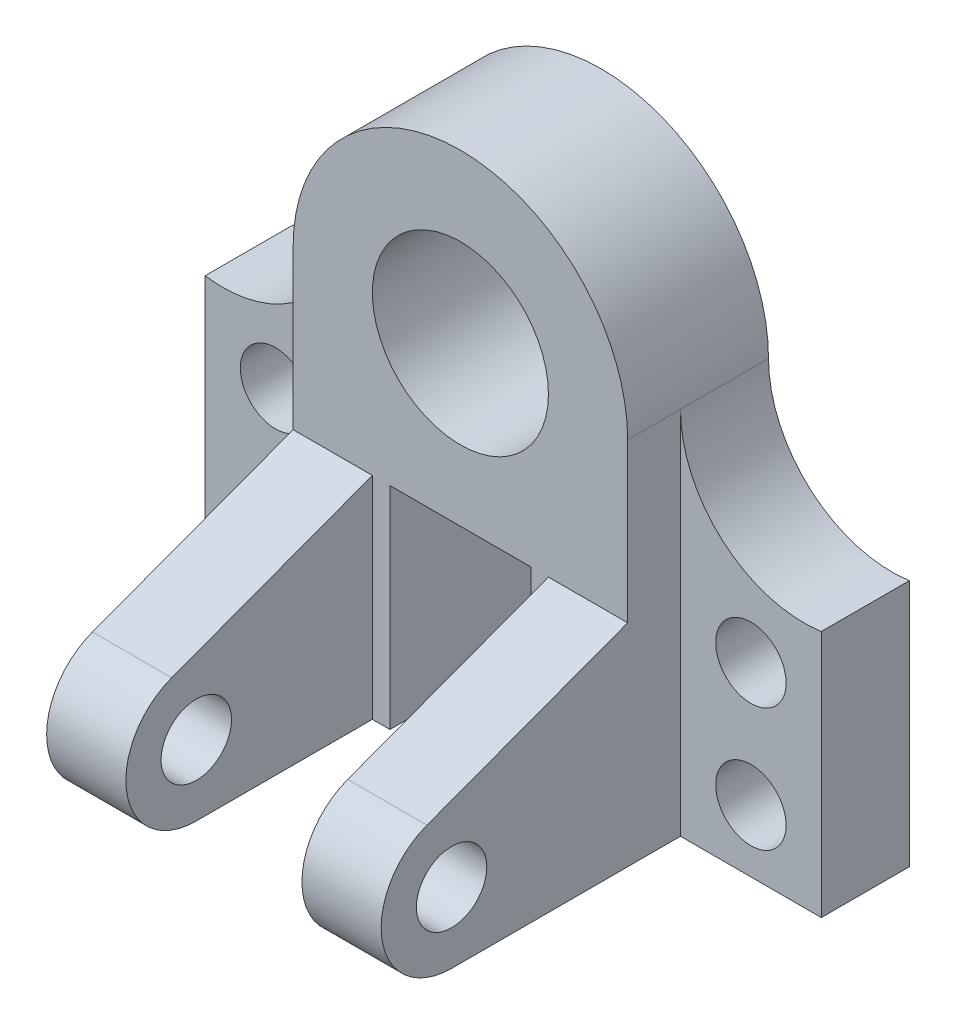
ISO-10303-21;
HEADER;
FILE_DESCRIPTION(('STEP AP214'),'2;1');
FILE_NAME('part.step','',(''),(''),'','','');
FILE_SCHEMA(('AUTOMOTIVE_DESIGN { 1 0 10303 214 1 1 1 1 }'));
ENDSEC;
DATA;
#1=APPLICATION_CONTEXT('core data for automotive mechanical design processes');
#2=APPLICATION_PROTOCOL_DEFINITION('international standard','automotive_design',2000,#1);
#3=PRODUCT_CONTEXT('',#1,'mechanical');
#4=PRODUCT('Part','Part','',(#3));
#5=PRODUCT_RELATED_PRODUCT_CATEGORY('part','',(#4));
#6=PRODUCT_DEFINITION_FORMATION('','',#4);
#7=PRODUCT_DEFINITION_CONTEXT('part definition',#1,'design');
#8=PRODUCT_DEFINITION('design','',#6,#7);
#9=PRODUCT_DEFINITION_SHAPE('','',#8);
#10=(LENGTH_UNIT() NAMED_UNIT(*) SI_UNIT(.MILLI.,.METRE.));
#11=(NAMED_UNIT(*) PLANE_ANGLE_UNIT() SI_UNIT($,.RADIAN.));
#12=(NAMED_UNIT(*) SI_UNIT($,.STERADIAN.) SOLID_ANGLE_UNIT());
#13=UNCERTAINTY_MEASURE_WITH_UNIT(LENGTH_MEASURE(1.E-05),#10,'distance_accuracy_value','');
#14=(GEOMETRIC_REPRESENTATION_CONTEXT(3) GLOBAL_UNCERTAINTY_ASSIGNED_CONTEXT((#13)) GLOBAL_UNIT_ASSIGNED_CONTEXT((#10,
#11,#12)) REPRESENTATION_CONTEXT('',''));
#15=CARTESIAN_POINT('',(0.,0.,0.));
#16=DIRECTION('',(0.,0.,1.));
#17=DIRECTION('',(1.,0.,0.));
#18=AXIS2_PLACEMENT_3D('',#15,#16,#17);
#19=CARTESIAN_POINT('',(-38.,-84.,32.));
#20=DIRECTION('',(0.,1.,0.));
#21=DIRECTION('',(0.,0.,1.));
#22=AXIS2_PLACEMENT_3D('',#19,#20,#21);
#23=PLANE('',#22);
#24=DIRECTION('',(1.,0.,0.));
#25=VECTOR('',#24,1.);
#26=CARTESIAN_POINT('',(-38.,-84.,0.));
#27=LINE('',#26,#25);
#28=CARTESIAN_POINT('',(-70.,-84.,0.));
#29=VERTEX_POINT('',#28);
#30=CARTESIAN_POINT('',(-16.,-84.,0.));
#31=VERTEX_POINT('',#30);
#32=EDGE_CURVE('E192',#29,#31,#27,.T.);
#33=ORIENTED_EDGE('',*,*,#32,.T.);
#34=DIRECTION('',(0.,0.,1.));
#35=VECTOR('',#34,1.);
#36=CARTESIAN_POINT('',(-16.,-84.,0.));
#37=LINE('',#36,#35);
#38=CARTESIAN_POINT('',(-16.,-84.,32.));
#39=VERTEX_POINT('',#38);
#40=EDGE_CURVE('E176',#31,#39,#37,.T.);
#41=ORIENTED_EDGE('',*,*,#40,.T.);
#42=DIRECTION('',(1.,0.,0.));
#43=VECTOR('',#42,1.);
#44=CARTESIAN_POINT('',(-38.,-84.,32.));
#45=LINE('',#44,#43);
#46=CARTESIAN_POINT('',(-20.,-84.,32.));
#47=VERTEX_POINT('',#46);
#48=EDGE_CURVE('E257',#47,#39,#45,.T.);
#49=ORIENTED_EDGE('',*,*,#48,.F.);
#50=DIRECTION('',(0.,0.,1.));
#51=VECTOR('',#50,1.);
#52=CARTESIAN_POINT('',(-20.,-84.,72.));
#53=LINE('',#52,#51);
#54=CARTESIAN_POINT('',(-20.,-84.,72.));
#55=VERTEX_POINT('',#54);
#56=EDGE_CURVE('E282',#47,#55,#53,.T.);
#57=ORIENTED_EDGE('',*,*,#56,.T.);
#58=DIRECTION('',(-1.,0.,0.));
#59=VECTOR('',#58,1.);
#60=CARTESIAN_POINT('',(-20.,-84.,72.));
#61=LINE('',#60,#59);
#62=CARTESIAN_POINT('',(-38.,-84.,72.));
#63=VERTEX_POINT('',#62);
#64=EDGE_CURVE('E223',#55,#63,#61,.T.);
#65=ORIENTED_EDGE('',*,*,#64,.T.);
#66=DIRECTION('',(0.,0.,-1.));
#67=VECTOR('',#66,1.);
#68=CARTESIAN_POINT('',(-38.,-84.,32.));
#69=LINE('',#68,#67);
#70=CARTESIAN_POINT('',(-38.,-84.,20.));
#71=VERTEX_POINT('',#70);
#72=EDGE_CURVE('E55',#63,#71,#69,.T.);
#73=ORIENTED_EDGE('',*,*,#72,.T.);
#74=DIRECTION('',(-1.,0.,0.));
#75=VECTOR('',#74,1.);
#76=CARTESIAN_POINT('',(-38.,-84.,20.));
#77=LINE('',#76,#75);
#78=CARTESIAN_POINT('',(-70.,-84.,20.));
#79=VERTEX_POINT('',#78);
#80=EDGE_CURVE('E218',#71,#79,#77,.T.);
#81=ORIENTED_EDGE('',*,*,#80,.T.);
#82=DIRECTION('',(0.,0.,-1.));
#83=VECTOR('',#82,1.);
#84=CARTESIAN_POINT('',(-70.,-84.,20.));
#85=LINE('',#84,#83);
#86=EDGE_CURVE('E200',#79,#29,#85,.T.);
#87=ORIENTED_EDGE('',*,*,#86,.T.);
#88=EDGE_LOOP('',(#33,#41,#49,#57,#65,#73,#81,#87));
#89=FACE_BOUND('',#88,.T.);
#90=ADVANCED_FACE('F43',(#89),#23,.F.);
#91=CARTESIAN_POINT('',(-38.,0.,32.));
#92=DIRECTION('',(1.,0.,0.));
#93=DIRECTION('',(0.,1.,0.));
#94=AXIS2_PLACEMENT_3D('',#91,#92,#93);
#95=PLANE('',#94);
#96=CARTESIAN_POINT('',(-38.,-68.,72.));
#97=DIRECTION('',(-1.,0.,0.));
#98=DIRECTION('',(0.,-1.,0.));
#99=AXIS2_PLACEMENT_3D('',#96,#97,#98);
#100=CIRCLE('',#99,7.99999999999999);
#101=CARTESIAN_POINT('',(-38.,-76.,72.));
#102=VERTEX_POINT('',#101);
#103=EDGE_CURVE('E693',#102,#102,#100,.T.);
#104=ORIENTED_EDGE('',*,*,#103,.F.);
#105=EDGE_LOOP('',(#104));
#106=FACE_BOUND('',#105,.T.);
#107=DIRECTION('',(0.,-1.,0.));
#108=VECTOR('',#107,1.);
#109=CARTESIAN_POINT('',(-38.,0.,20.));
#110=LINE('',#109,#108);
#111=CARTESIAN_POINT('',(-38.,0.,20.));
#112=VERTEX_POINT('',#111);
#113=EDGE_CURVE('E229',#112,#71,#110,.T.);
#114=ORIENTED_EDGE('',*,*,#113,.T.);
#115=ORIENTED_EDGE('',*,*,#72,.F.);
#116=CARTESIAN_POINT('',(-38.,-68.,72.));
#117=DIRECTION('',(-1.,0.,0.));
#118=DIRECTION('',(0.,-1.,0.));
#119=AXIS2_PLACEMENT_3D('',#116,#117,#118);
#120=CIRCLE('',#119,16.);
#121=CARTESIAN_POINT('',(-38.,-53.0092438433205,77.5926049253436));
#122=VERTEX_POINT('',#121);
#123=EDGE_CURVE('E378',#63,#122,#120,.T.);
#124=ORIENTED_EDGE('',*,*,#123,.T.);
#125=DIRECTION('',(0.,0.349537807833973,-0.936922259792466));
#126=VECTOR('',#125,1.);
#127=CARTESIAN_POINT('',(-38.,-36.,32.));
#128=LINE('',#127,#126);
#129=CARTESIAN_POINT('',(-38.,-36.,32.));
#130=VERTEX_POINT('',#129);
#131=EDGE_CURVE('E274',#122,#130,#128,.T.);
#132=ORIENTED_EDGE('',*,*,#131,.T.);
#133=DIRECTION('',(0.,-1.,0.));
#134=VECTOR('',#133,1.);
#135=CARTESIAN_POINT('',(-38.,0.,32.));
#136=LINE('',#135,#134);
#137=CARTESIAN_POINT('',(-38.,0.,32.));
#138=VERTEX_POINT('',#137);
#139=EDGE_CURVE('E202',#138,#130,#136,.T.);
#140=ORIENTED_EDGE('',*,*,#139,.F.);
#141=DIRECTION('',(0.,0.,-1.));
#142=VECTOR('',#141,1.);
#143=CARTESIAN_POINT('',(-38.,0.,32.));
#144=LINE('',#143,#142);
#145=EDGE_CURVE('E11',#138,#112,#144,.T.);
#146=ORIENTED_EDGE('',*,*,#145,.T.);
#147=EDGE_LOOP('',(#114,#115,#124,#132,#140,#146));
#148=FACE_BOUND('',#147,.T.);
#149=ADVANCED_FACE('F272',(#106,#148),#95,.F.);
#150=CARTESIAN_POINT('',(0.,0.,32.));
#151=DIRECTION('',(0.,0.,-1.));
#152=DIRECTION('',(-1.,0.,0.));
#153=AXIS2_PLACEMENT_3D('',#150,#151,#152);
#154=CYLINDRICAL_SURFACE('',#153,38.);
#155=CARTESIAN_POINT('',(0.,0.,0.));
#156=DIRECTION('',(0.,0.,1.));
#157=DIRECTION('',(1.,0.,0.));
#158=AXIS2_PLACEMENT_3D('',#155,#156,#157);
#159=CIRCLE('',#158,38.);
#160=CARTESIAN_POINT('',(38.,-2.57695444354224E-13,0.));
#161=VERTEX_POINT('',#160);
#162=CARTESIAN_POINT('',(-38.,0.,0.));
#163=VERTEX_POINT('',#162);
#164=EDGE_CURVE('E207',#161,#163,#159,.T.);
#165=ORIENTED_EDGE('',*,*,#164,.T.);
#166=DIRECTION('',(0.,0.,-1.));
#167=VECTOR('',#166,1.);
#168=CARTESIAN_POINT('',(-38.,0.,20.));
#169=LINE('',#168,#167);
#170=EDGE_CURVE('E250',#112,#163,#169,.T.);
#171=ORIENTED_EDGE('',*,*,#170,.F.);
#172=ORIENTED_EDGE('',*,*,#145,.F.);
#173=CARTESIAN_POINT('',(0.,0.,32.));
#174=DIRECTION('',(0.,0.,1.));
#175=DIRECTION('',(1.,0.,0.));
#176=AXIS2_PLACEMENT_3D('',#173,#174,#175);
#177=CIRCLE('',#176,38.);
#178=CARTESIAN_POINT('',(38.,0.,32.));
#179=VERTEX_POINT('',#178);
#180=EDGE_CURVE('E197',#179,#138,#177,.T.);
#181=ORIENTED_EDGE('',*,*,#180,.F.);
#182=DIRECTION('',(0.,0.,-1.));
#183=VECTOR('',#182,1.);
#184=CARTESIAN_POINT('',(38.,0.,32.));
#185=LINE('',#184,#183);
#186=CARTESIAN_POINT('',(38.,0.,20.));
#187=VERTEX_POINT('',#186);
#188=EDGE_CURVE('E208',#179,#187,#185,.T.);
#189=ORIENTED_EDGE('',*,*,#188,.T.);
#190=DIRECTION('',(0.,0.,-1.));
#191=VECTOR('',#190,1.);
#192=CARTESIAN_POINT('',(38.,-2.57695444354224E-13,20.));
#193=LINE('',#192,#191);
#194=EDGE_CURVE('E297',#187,#161,#193,.T.);
#195=ORIENTED_EDGE('',*,*,#194,.T.);
#196=EDGE_LOOP('',(#165,#171,#172,#181,#189,#195));
#197=FACE_BOUND('',#196,.T.);
#198=ADVANCED_FACE('F44',(#197),#154,.T.);
#199=CARTESIAN_POINT('',(16.,-84.,32.));
#200=VERTEX_POINT('',#199);
#201=CARTESIAN_POINT('',(20.,-84.,32.));
#202=VERTEX_POINT('',#201);
#203=EDGE_CURVE('E253',#200,#202,#45,.T.);
#204=ORIENTED_EDGE('',*,*,#203,.F.);
#205=DIRECTION('',(0.,0.,1.));
#206=VECTOR('',#205,1.);
#207=CARTESIAN_POINT('',(16.,-84.,0.));
#208=LINE('',#207,#206);
#209=CARTESIAN_POINT('',(16.,-84.,0.));
#210=VERTEX_POINT('',#209);
#211=EDGE_CURVE('E187',#210,#200,#208,.T.);
#212=ORIENTED_EDGE('',*,*,#211,.F.);
#213=CARTESIAN_POINT('',(70.,-84.,0.));
#214=VERTEX_POINT('',#213);
#215=EDGE_CURVE('E203',#210,#214,#27,.T.);
#216=ORIENTED_EDGE('',*,*,#215,.T.);
#217=DIRECTION('',(0.,0.,-1.));
#218=VECTOR('',#217,1.);
#219=CARTESIAN_POINT('',(70.,-84.,20.));
#220=LINE('',#219,#218);
#221=CARTESIAN_POINT('',(70.,-84.,20.));
#222=VERTEX_POINT('',#221);
#223=EDGE_CURVE('E242',#222,#214,#220,.T.);
#224=ORIENTED_EDGE('',*,*,#223,.F.);
#225=DIRECTION('',(-1.,0.,0.));
#226=VECTOR('',#225,1.);
#227=CARTESIAN_POINT('',(38.,-84.,20.));
#228=LINE('',#227,#226);
#229=CARTESIAN_POINT('',(38.,-84.,20.));
#230=VERTEX_POINT('',#229);
#231=EDGE_CURVE('E300',#222,#230,#228,.T.);
#232=ORIENTED_EDGE('',*,*,#231,.T.);
#233=DIRECTION('',(0.,0.,-1.));
#234=VECTOR('',#233,1.);
#235=CARTESIAN_POINT('',(38.,-84.,32.));
#236=LINE('',#235,#234);
#237=CARTESIAN_POINT('',(38.,-84.,72.));
#238=VERTEX_POINT('',#237);
#239=EDGE_CURVE('E214',#238,#230,#236,.T.);
#240=ORIENTED_EDGE('',*,*,#239,.F.);
#241=DIRECTION('',(1.,0.,0.));
#242=VECTOR('',#241,1.);
#243=CARTESIAN_POINT('',(20.,-84.,72.));
#244=LINE('',#243,#242);
#245=CARTESIAN_POINT('',(20.,-84.,72.));
#246=VERTEX_POINT('',#245);
#247=EDGE_CURVE('E362',#246,#238,#244,.T.);
#248=ORIENTED_EDGE('',*,*,#247,.F.);
#249=DIRECTION('',(0.,0.,-1.));
#250=VECTOR('',#249,1.);
#251=CARTESIAN_POINT('',(20.,-84.,72.));
#252=LINE('',#251,#250);
#253=EDGE_CURVE('E355',#246,#202,#252,.T.);
#254=ORIENTED_EDGE('',*,*,#253,.T.);
#255=EDGE_LOOP('',(#204,#212,#216,#224,#232,#240,#248,#254));
#256=FACE_BOUND('',#255,.T.);
#257=ADVANCED_FACE('F331',(#256),#23,.F.);
#258=CARTESIAN_POINT('',(38.,-84.,32.));
#259=DIRECTION('',(-1.,0.,0.));
#260=DIRECTION('',(0.,-1.,0.));
#261=AXIS2_PLACEMENT_3D('',#258,#259,#260);
#262=PLANE('',#261);
#263=CARTESIAN_POINT('',(38.,-68.,72.));
#264=DIRECTION('',(-1.,0.,0.));
#265=DIRECTION('',(0.,-1.,0.));
#266=AXIS2_PLACEMENT_3D('',#263,#264,#265);
#267=CIRCLE('',#266,7.99999999999999);
#268=CARTESIAN_POINT('',(38.,-76.,72.));
#269=VERTEX_POINT('',#268);
#270=EDGE_CURVE('E701',#269,#269,#267,.T.);
#271=ORIENTED_EDGE('',*,*,#270,.T.);
#272=EDGE_LOOP('',(#271));
#273=FACE_BOUND('',#272,.T.);
#274=ORIENTED_EDGE('',*,*,#239,.T.);
#275=DIRECTION('',(0.,1.,0.));
#276=VECTOR('',#275,1.);
#277=CARTESIAN_POINT('',(38.,-2.65352581752078E-13,20.));
#278=LINE('',#277,#276);
#279=EDGE_CURVE('E270',#230,#187,#278,.T.);
#280=ORIENTED_EDGE('',*,*,#279,.T.);
#281=ORIENTED_EDGE('',*,*,#188,.F.);
#282=DIRECTION('',(0.,1.,0.));
#283=VECTOR('',#282,1.);
#284=CARTESIAN_POINT('',(38.,-84.,32.));
#285=LINE('',#284,#283);
#286=CARTESIAN_POINT('',(38.,-36.,32.));
#287=VERTEX_POINT('',#286);
#288=EDGE_CURVE('E211',#287,#179,#285,.T.);
#289=ORIENTED_EDGE('',*,*,#288,.F.);
#290=DIRECTION('',(0.,-0.349537807833973,0.936922259792466));
#291=VECTOR('',#290,1.);
#292=CARTESIAN_POINT('',(38.,-36.,32.));
#293=LINE('',#292,#291);
#294=CARTESIAN_POINT('',(38.,-53.0092438433205,77.5926049253436));
#295=VERTEX_POINT('',#294);
#296=EDGE_CURVE('E372',#287,#295,#293,.T.);
#297=ORIENTED_EDGE('',*,*,#296,.T.);
#298=CARTESIAN_POINT('',(38.,-68.,72.));
#299=DIRECTION('',(1.,0.,0.));
#300=DIRECTION('',(0.,1.,0.));
#301=AXIS2_PLACEMENT_3D('',#298,#299,#300);
#302=CIRCLE('',#301,16.);
#303=EDGE_CURVE('E371',#295,#238,#302,.T.);
#304=ORIENTED_EDGE('',*,*,#303,.T.);
#305=EDGE_LOOP('',(#274,#280,#281,#289,#297,#304));
#306=FACE_BOUND('',#305,.T.);
#307=ADVANCED_FACE('F262',(#273,#306),#262,.F.);
#308=CARTESIAN_POINT('',(0.,0.,32.));
#309=DIRECTION('',(0.,0.,1.));
#310=DIRECTION('',(1.,0.,0.));
#311=AXIS2_PLACEMENT_3D('',#308,#309,#310);
#312=PLANE('',#311);
#313=CARTESIAN_POINT('',(0.,0.,32.));
#314=DIRECTION('',(0.,0.,1.));
#315=DIRECTION('',(1.,0.,0.));
#316=AXIS2_PLACEMENT_3D('',#313,#314,#315);
#317=CIRCLE('',#316,20.);
#318=CARTESIAN_POINT('',(20.,0.,32.));
#319=VERTEX_POINT('',#318);
#320=EDGE_CURVE('E686',#319,#319,#317,.T.);
#321=ORIENTED_EDGE('',*,*,#320,.F.);
#322=EDGE_LOOP('',(#321));
#323=FACE_BOUND('',#322,.T.);
#324=DIRECTION('',(0.,-1.,0.));
#325=VECTOR('',#324,1.);
#326=CARTESIAN_POINT('',(-16.,-84.,32.));
#327=LINE('',#326,#325);
#328=CARTESIAN_POINT('',(-16.,-36.,32.));
#329=VERTEX_POINT('',#328);
#330=EDGE_CURVE('E181',#329,#39,#327,.T.);
#331=ORIENTED_EDGE('',*,*,#330,.F.);
#332=DIRECTION('',(-1.,0.,0.));
#333=VECTOR('',#332,1.);
#334=CARTESIAN_POINT('',(-16.,-36.,32.));
#335=LINE('',#334,#333);
#336=CARTESIAN_POINT('',(16.,-36.,32.));
#337=VERTEX_POINT('',#336);
#338=EDGE_CURVE('E193',#337,#329,#335,.T.);
#339=ORIENTED_EDGE('',*,*,#338,.F.);
#340=DIRECTION('',(0.,1.,0.));
#341=VECTOR('',#340,1.);
#342=CARTESIAN_POINT('',(16.,-84.,32.));
#343=LINE('',#342,#341);
#344=EDGE_CURVE('E358',#200,#337,#343,.T.);
#345=ORIENTED_EDGE('',*,*,#344,.F.);
#346=ORIENTED_EDGE('',*,*,#203,.T.);
#347=DIRECTION('',(0.,1.,0.));
#348=VECTOR('',#347,1.);
#349=CARTESIAN_POINT('',(20.,-84.,32.));
#350=LINE('',#349,#348);
#351=CARTESIAN_POINT('',(20.,-36.,32.));
#352=VERTEX_POINT('',#351);
#353=EDGE_CURVE('E66',#202,#352,#350,.T.);
#354=ORIENTED_EDGE('',*,*,#353,.T.);
#355=DIRECTION('',(1.,0.,0.));
#356=VECTOR('',#355,1.);
#357=CARTESIAN_POINT('',(20.,-36.,32.));
#358=LINE('',#357,#356);
#359=EDGE_CURVE('E264',#352,#287,#358,.T.);
#360=ORIENTED_EDGE('',*,*,#359,.T.);
#361=ORIENTED_EDGE('',*,*,#288,.T.);
#362=ORIENTED_EDGE('',*,*,#180,.T.);
#363=ORIENTED_EDGE('',*,*,#139,.T.);
#364=DIRECTION('',(-1.,0.,0.));
#365=VECTOR('',#364,1.);
#366=CARTESIAN_POINT('',(-20.,-36.,32.));
#367=LINE('',#366,#365);
#368=CARTESIAN_POINT('',(-20.,-36.,32.));
#369=VERTEX_POINT('',#368);
#370=EDGE_CURVE('E280',#369,#130,#367,.T.);
#371=ORIENTED_EDGE('',*,*,#370,.F.);
#372=DIRECTION('',(0.,-1.,0.));
#373=VECTOR('',#372,1.);
#374=CARTESIAN_POINT('',(-20.,-84.,32.));
#375=LINE('',#374,#373);
#376=EDGE_CURVE('E279',#369,#47,#375,.T.);
#377=ORIENTED_EDGE('',*,*,#376,.T.);
#378=ORIENTED_EDGE('',*,*,#48,.T.);
#379=EDGE_LOOP('',(#331,#339,#345,#346,#354,#360,#361,#362,#363,#371,#377,#378));
#380=FACE_BOUND('',#379,.T.);
#381=ADVANCED_FACE('F259',(#323,#380),#312,.T.);
#382=CARTESIAN_POINT('',(0.,0.,0.));
#383=DIRECTION('',(0.,0.,1.));
#384=DIRECTION('',(1.,0.,0.));
#385=AXIS2_PLACEMENT_3D('',#382,#383,#384);
#386=PLANE('',#385);
#387=CARTESIAN_POINT('',(0.,0.,0.));
#388=DIRECTION('',(0.,0.,1.));
#389=DIRECTION('',(1.,0.,0.));
#390=AXIS2_PLACEMENT_3D('',#387,#388,#389);
#391=CIRCLE('',#390,20.);
#392=CARTESIAN_POINT('',(20.,0.,0.));
#393=VERTEX_POINT('',#392);
#394=EDGE_CURVE('E687',#393,#393,#391,.T.);
#395=ORIENTED_EDGE('',*,*,#394,.T.);
#396=EDGE_LOOP('',(#395));
#397=FACE_BOUND('',#396,.T.);
#398=CARTESIAN_POINT('',(-54.,-69.856406460551,0.));
#399=DIRECTION('',(0.,0.,1.));
#400=DIRECTION('',(1.,0.,0.));
#401=AXIS2_PLACEMENT_3D('',#398,#399,#400);
#402=CIRCLE('',#401,8.);
#403=CARTESIAN_POINT('',(-46.,-69.856406460551,0.));
#404=VERTEX_POINT('',#403);
#405=EDGE_CURVE('E712',#404,#404,#402,.T.);
#406=ORIENTED_EDGE('',*,*,#405,.T.);
#407=EDGE_LOOP('',(#406));
#408=FACE_BOUND('',#407,.T.);
#409=CARTESIAN_POINT('',(54.,-41.856406460551,0.));
#410=DIRECTION('',(0.,0.,1.));
#411=DIRECTION('',(1.,0.,0.));
#412=AXIS2_PLACEMENT_3D('',#409,#410,#411);
#413=CIRCLE('',#412,8.);
#414=CARTESIAN_POINT('',(62.,-41.856406460551,0.));
#415=VERTEX_POINT('',#414);
#416=EDGE_CURVE('E720',#415,#415,#413,.T.);
#417=ORIENTED_EDGE('',*,*,#416,.T.);
#418=EDGE_LOOP('',(#417));
#419=FACE_BOUND('',#418,.T.);
#420=CARTESIAN_POINT('',(54.,-69.856406460551,0.));
#421=DIRECTION('',(0.,0.,1.));
#422=DIRECTION('',(1.,0.,0.));
#423=AXIS2_PLACEMENT_3D('',#420,#421,#422);
#424=CIRCLE('',#423,8.);
#425=CARTESIAN_POINT('',(62.,-69.856406460551,0.));
#426=VERTEX_POINT('',#425);
#427=EDGE_CURVE('E704',#426,#426,#424,.T.);
#428=ORIENTED_EDGE('',*,*,#427,.T.);
#429=EDGE_LOOP('',(#428));
#430=FACE_BOUND('',#429,.T.);
#431=CARTESIAN_POINT('',(-54.,-41.856406460551,0.));
#432=DIRECTION('',(0.,0.,1.));
#433=DIRECTION('',(1.,0.,0.));
#434=AXIS2_PLACEMENT_3D('',#431,#432,#433);
#435=CIRCLE('',#434,8.);
#436=CARTESIAN_POINT('',(-46.,-41.856406460551,0.));
#437=VERTEX_POINT('',#436);
#438=EDGE_CURVE('E721',#437,#437,#435,.T.);
#439=ORIENTED_EDGE('',*,*,#438,.T.);
#440=EDGE_LOOP('',(#439));
#441=FACE_BOUND('',#440,.T.);
#442=DIRECTION('',(-1.,0.,0.));
#443=VECTOR('',#442,1.);
#444=CARTESIAN_POINT('',(-16.,-36.,0.));
#445=LINE('',#444,#443);
#446=CARTESIAN_POINT('',(16.,-36.,0.));
#447=VERTEX_POINT('',#446);
#448=CARTESIAN_POINT('',(-16.,-36.,0.));
#449=VERTEX_POINT('',#448);
#450=EDGE_CURVE('E56',#447,#449,#445,.T.);
#451=ORIENTED_EDGE('',*,*,#450,.T.);
#452=DIRECTION('',(0.,-1.,0.));
#453=VECTOR('',#452,1.);
#454=CARTESIAN_POINT('',(-16.,-84.,0.));
#455=LINE('',#454,#453);
#456=EDGE_CURVE('E177',#449,#31,#455,.T.);
#457=ORIENTED_EDGE('',*,*,#456,.T.);
#458=ORIENTED_EDGE('',*,*,#32,.F.);
#459=DIRECTION('',(0.,1.,0.));
#460=VECTOR('',#459,1.);
#461=CARTESIAN_POINT('',(-70.,-84.,0.));
#462=LINE('',#461,#460);
#463=CARTESIAN_POINT('',(-70.,-27.712812921102,0.));
#464=VERTEX_POINT('',#463);
#465=EDGE_CURVE('E245',#29,#464,#462,.T.);
#466=ORIENTED_EDGE('',*,*,#465,.T.);
#467=CARTESIAN_POINT('',(-66.,0.,0.));
#468=DIRECTION('',(0.,0.,1.));
#469=DIRECTION('',(-1.,0.,0.));
#470=AXIS2_PLACEMENT_3D('',#467,#468,#469);
#471=CIRCLE('',#470,28.);
#472=EDGE_CURVE('E240',#464,#163,#471,.T.);
#473=ORIENTED_EDGE('',*,*,#472,.T.);
#474=ORIENTED_EDGE('',*,*,#164,.F.);
#475=CARTESIAN_POINT('',(66.,0.,0.));
#476=DIRECTION('',(0.,0.,1.));
#477=DIRECTION('',(1.,0.,0.));
#478=AXIS2_PLACEMENT_3D('',#475,#476,#477);
#479=CIRCLE('',#478,28.);
#480=CARTESIAN_POINT('',(70.,-27.712812921102,0.));
#481=VERTEX_POINT('',#480);
#482=EDGE_CURVE('E285',#161,#481,#479,.T.);
#483=ORIENTED_EDGE('',*,*,#482,.T.);
#484=DIRECTION('',(0.,-1.,0.));
#485=VECTOR('',#484,1.);
#486=CARTESIAN_POINT('',(70.,-84.,0.));
#487=LINE('',#486,#485);
#488=EDGE_CURVE('E293',#481,#214,#487,.T.);
#489=ORIENTED_EDGE('',*,*,#488,.T.);
#490=ORIENTED_EDGE('',*,*,#215,.F.);
#491=DIRECTION('',(0.,1.,0.));
#492=VECTOR('',#491,1.);
#493=CARTESIAN_POINT('',(16.,-84.,0.));
#494=LINE('',#493,#492);
#495=EDGE_CURVE('E191',#210,#447,#494,.T.);
#496=ORIENTED_EDGE('',*,*,#495,.T.);
#497=EDGE_LOOP('',(#451,#457,#458,#466,#473,#474,#483,#489,#490,#496));
#498=FACE_BOUND('',#497,.T.);
#499=ADVANCED_FACE('F186',(#397,#408,#419,#430,#441,#498),#386,.F.);
#500=CARTESIAN_POINT('',(-66.,0.,20.));
#501=DIRECTION('',(0.,0.,-1.));
#502=DIRECTION('',(-1.,0.,0.));
#503=AXIS2_PLACEMENT_3D('',#500,#501,#502);
#504=CYLINDRICAL_SURFACE('',#503,28.);
#505=ORIENTED_EDGE('',*,*,#472,.F.);
#506=DIRECTION('',(0.,0.,-1.));
#507=VECTOR('',#506,1.);
#508=CARTESIAN_POINT('',(-70.,-27.712812921102,20.));
#509=LINE('',#508,#507);
#510=CARTESIAN_POINT('',(-70.,-27.712812921102,20.));
#511=VERTEX_POINT('',#510);
#512=EDGE_CURVE('E249',#511,#464,#509,.T.);
#513=ORIENTED_EDGE('',*,*,#512,.F.);
#514=CARTESIAN_POINT('',(-66.,0.,20.));
#515=DIRECTION('',(0.,0.,1.));
#516=DIRECTION('',(-1.,0.,0.));
#517=AXIS2_PLACEMENT_3D('',#514,#515,#516);
#518=CIRCLE('',#517,28.);
#519=EDGE_CURVE('E232',#511,#112,#518,.T.);
#520=ORIENTED_EDGE('',*,*,#519,.T.);
#521=ORIENTED_EDGE('',*,*,#170,.T.);
#522=EDGE_LOOP('',(#505,#513,#520,#521));
#523=FACE_BOUND('',#522,.T.);
#524=ADVANCED_FACE('F317',(#523),#504,.F.);
#525=CARTESIAN_POINT('',(-70.,-84.,20.));
#526=DIRECTION('',(-1.,0.,0.));
#527=DIRECTION('',(0.,0.,1.));
#528=AXIS2_PLACEMENT_3D('',#525,#526,#527);
#529=PLANE('',#528);
#530=ORIENTED_EDGE('',*,*,#465,.F.);
#531=ORIENTED_EDGE('',*,*,#86,.F.);
#532=DIRECTION('',(0.,1.,0.));
#533=VECTOR('',#532,1.);
#534=CARTESIAN_POINT('',(-70.,-84.,20.));
#535=LINE('',#534,#533);
#536=EDGE_CURVE('E231',#79,#511,#535,.T.);
#537=ORIENTED_EDGE('',*,*,#536,.T.);
#538=ORIENTED_EDGE('',*,*,#512,.T.);
#539=EDGE_LOOP('',(#530,#531,#537,#538));
#540=FACE_BOUND('',#539,.T.);
#541=ADVANCED_FACE('F319',(#540),#529,.T.);
#542=CARTESIAN_POINT('',(-66.,0.,20.));
#543=DIRECTION('',(0.,0.,-1.));
#544=DIRECTION('',(-1.,0.,0.));
#545=AXIS2_PLACEMENT_3D('',#542,#543,#544);
#546=PLANE('',#545);
#547=CARTESIAN_POINT('',(-54.,-69.856406460551,20.));
#548=DIRECTION('',(0.,0.,1.));
#549=DIRECTION('',(1.,0.,0.));
#550=AXIS2_PLACEMENT_3D('',#547,#548,#549);
#551=CIRCLE('',#550,8.);
#552=CARTESIAN_POINT('',(-46.,-69.856406460551,20.));
#553=VERTEX_POINT('',#552);
#554=EDGE_CURVE('E713',#553,#553,#551,.T.);
#555=ORIENTED_EDGE('',*,*,#554,.F.);
#556=EDGE_LOOP('',(#555));
#557=FACE_BOUND('',#556,.T.);
#558=CARTESIAN_POINT('',(-54.,-41.856406460551,20.));
#559=DIRECTION('',(0.,0.,1.));
#560=DIRECTION('',(1.,0.,0.));
#561=AXIS2_PLACEMENT_3D('',#558,#559,#560);
#562=CIRCLE('',#561,8.);
#563=CARTESIAN_POINT('',(-46.,-41.856406460551,20.));
#564=VERTEX_POINT('',#563);
#565=EDGE_CURVE('E711',#564,#564,#562,.T.);
#566=ORIENTED_EDGE('',*,*,#565,.F.);
#567=EDGE_LOOP('',(#566));
#568=FACE_BOUND('',#567,.T.);
#569=ORIENTED_EDGE('',*,*,#113,.F.);
#570=ORIENTED_EDGE('',*,*,#519,.F.);
#571=ORIENTED_EDGE('',*,*,#536,.F.);
#572=ORIENTED_EDGE('',*,*,#80,.F.);
#573=EDGE_LOOP('',(#569,#570,#571,#572));
#574=FACE_BOUND('',#573,.T.);
#575=ADVANCED_FACE('F226',(#557,#568,#574),#546,.F.);
#576=CARTESIAN_POINT('',(70.,-84.,20.));
#577=DIRECTION('',(1.,0.,0.));
#578=DIRECTION('',(0.,1.,0.));
#579=AXIS2_PLACEMENT_3D('',#576,#577,#578);
#580=PLANE('',#579);
#581=ORIENTED_EDGE('',*,*,#488,.F.);
#582=DIRECTION('',(0.,0.,-1.));
#583=VECTOR('',#582,1.);
#584=CARTESIAN_POINT('',(70.,-27.712812921102,20.));
#585=LINE('',#584,#583);
#586=CARTESIAN_POINT('',(70.,-27.712812921102,20.));
#587=VERTEX_POINT('',#586);
#588=EDGE_CURVE('E310',#587,#481,#585,.T.);
#589=ORIENTED_EDGE('',*,*,#588,.F.);
#590=DIRECTION('',(0.,-1.,0.));
#591=VECTOR('',#590,1.);
#592=CARTESIAN_POINT('',(70.,-84.,20.));
#593=LINE('',#592,#591);
#594=EDGE_CURVE('E295',#587,#222,#593,.T.);
#595=ORIENTED_EDGE('',*,*,#594,.T.);
#596=ORIENTED_EDGE('',*,*,#223,.T.);
#597=EDGE_LOOP('',(#581,#589,#595,#596));
#598=FACE_BOUND('',#597,.T.);
#599=ADVANCED_FACE('F329',(#598),#580,.T.);
#600=CARTESIAN_POINT('',(66.,0.,20.));
#601=DIRECTION('',(0.,0.,-1.));
#602=DIRECTION('',(-1.,0.,0.));
#603=AXIS2_PLACEMENT_3D('',#600,#601,#602);
#604=CYLINDRICAL_SURFACE('',#603,28.);
#605=ORIENTED_EDGE('',*,*,#482,.F.);
#606=ORIENTED_EDGE('',*,*,#194,.F.);
#607=CARTESIAN_POINT('',(66.,0.,20.));
#608=DIRECTION('',(0.,0.,1.));
#609=DIRECTION('',(1.,0.,0.));
#610=AXIS2_PLACEMENT_3D('',#607,#608,#609);
#611=CIRCLE('',#610,28.);
#612=EDGE_CURVE('E289',#187,#587,#611,.T.);
#613=ORIENTED_EDGE('',*,*,#612,.T.);
#614=ORIENTED_EDGE('',*,*,#588,.T.);
#615=EDGE_LOOP('',(#605,#606,#613,#614));
#616=FACE_BOUND('',#615,.T.);
#617=ADVANCED_FACE('F311',(#616),#604,.F.);
#618=CARTESIAN_POINT('',(66.,0.,20.));
#619=DIRECTION('',(0.,0.,1.));
#620=DIRECTION('',(1.,0.,0.));
#621=AXIS2_PLACEMENT_3D('',#618,#619,#620);
#622=PLANE('',#621);
#623=CARTESIAN_POINT('',(54.,-41.856406460551,20.));
#624=DIRECTION('',(0.,0.,1.));
#625=DIRECTION('',(1.,0.,0.));
#626=AXIS2_PLACEMENT_3D('',#623,#624,#625);
#627=CIRCLE('',#626,8.);
#628=CARTESIAN_POINT('',(62.,-41.856406460551,20.));
#629=VERTEX_POINT('',#628);
#630=EDGE_CURVE('E709',#629,#629,#627,.T.);
#631=ORIENTED_EDGE('',*,*,#630,.F.);
#632=EDGE_LOOP('',(#631));
#633=FACE_BOUND('',#632,.T.);
#634=CARTESIAN_POINT('',(54.,-69.856406460551,20.));
#635=DIRECTION('',(0.,0.,1.));
#636=DIRECTION('',(1.,0.,0.));
#637=AXIS2_PLACEMENT_3D('',#634,#635,#636);
#638=CIRCLE('',#637,8.);
#639=CARTESIAN_POINT('',(62.,-69.856406460551,20.));
#640=VERTEX_POINT('',#639);
#641=EDGE_CURVE('E703',#640,#640,#638,.T.);
#642=ORIENTED_EDGE('',*,*,#641,.F.);
#643=EDGE_LOOP('',(#642));
#644=FACE_BOUND('',#643,.T.);
#645=ORIENTED_EDGE('',*,*,#279,.F.);
#646=ORIENTED_EDGE('',*,*,#231,.F.);
#647=ORIENTED_EDGE('',*,*,#594,.F.);
#648=ORIENTED_EDGE('',*,*,#612,.F.);
#649=EDGE_LOOP('',(#645,#646,#647,#648));
#650=FACE_BOUND('',#649,.T.);
#651=ADVANCED_FACE('F407',(#633,#644,#650),#622,.T.);
#652=CARTESIAN_POINT('',(-20.,-68.,72.));
#653=DIRECTION('',(-1.,0.,0.));
#654=DIRECTION('',(0.,-1.,0.));
#655=AXIS2_PLACEMENT_3D('',#652,#653,#654);
#656=CYLINDRICAL_SURFACE('',#655,16.);
#657=ORIENTED_EDGE('',*,*,#123,.F.);
#658=ORIENTED_EDGE('',*,*,#64,.F.);
#659=CARTESIAN_POINT('',(-20.,-68.,72.));
#660=DIRECTION('',(-1.,0.,0.));
#661=DIRECTION('',(0.,-1.,0.));
#662=AXIS2_PLACEMENT_3D('',#659,#660,#661);
#663=CIRCLE('',#662,16.);
#664=CARTESIAN_POINT('',(-20.,-53.0092438433205,77.5926049253436));
#665=VERTEX_POINT('',#664);
#666=EDGE_CURVE('E384',#55,#665,#663,.T.);
#667=ORIENTED_EDGE('',*,*,#666,.T.);
#668=DIRECTION('',(-1.,0.,0.));
#669=VECTOR('',#668,1.);
#670=CARTESIAN_POINT('',(-20.,-53.0092438433205,77.5926049253436));
#671=LINE('',#670,#669);
#672=EDGE_CURVE('E284',#665,#122,#671,.T.);
#673=ORIENTED_EDGE('',*,*,#672,.T.);
#674=EDGE_LOOP('',(#657,#658,#667,#673));
#675=FACE_BOUND('',#674,.T.);
#676=ADVANCED_FACE('F394',(#675),#656,.T.);
#677=CARTESIAN_POINT('',(-20.,-36.,32.));
#678=DIRECTION('',(0.,0.936922259792466,0.349537807833973));
#679=DIRECTION('',(0.,-0.349537807833973,0.936922259792466));
#680=AXIS2_PLACEMENT_3D('',#677,#678,#679);
#681=PLANE('',#680);
#682=ORIENTED_EDGE('',*,*,#131,.F.);
#683=ORIENTED_EDGE('',*,*,#672,.F.);
#684=DIRECTION('',(0.,0.349537807833973,-0.936922259792466));
#685=VECTOR('',#684,1.);
#686=CARTESIAN_POINT('',(-20.,-36.,32.));
#687=LINE('',#686,#685);
#688=EDGE_CURVE('E387',#665,#369,#687,.T.);
#689=ORIENTED_EDGE('',*,*,#688,.T.);
#690=ORIENTED_EDGE('',*,*,#370,.T.);
#691=EDGE_LOOP('',(#682,#683,#689,#690));
#692=FACE_BOUND('',#691,.T.);
#693=ADVANCED_FACE('F393',(#692),#681,.T.);
#694=CARTESIAN_POINT('',(-20.,-68.,72.));
#695=DIRECTION('',(-1.,0.,0.));
#696=DIRECTION('',(0.,-1.,0.));
#697=AXIS2_PLACEMENT_3D('',#694,#695,#696);
#698=PLANE('',#697);
#699=CARTESIAN_POINT('',(-20.,-68.,72.));
#700=DIRECTION('',(-1.,0.,0.));
#701=DIRECTION('',(0.,-1.,0.));
#702=AXIS2_PLACEMENT_3D('',#699,#700,#701);
#703=CIRCLE('',#702,7.99999999999999);
#704=CARTESIAN_POINT('',(-20.,-76.,72.));
#705=VERTEX_POINT('',#704);
#706=EDGE_CURVE('E698',#705,#705,#703,.T.);
#707=ORIENTED_EDGE('',*,*,#706,.T.);
#708=EDGE_LOOP('',(#707));
#709=FACE_BOUND('',#708,.T.);
#710=ORIENTED_EDGE('',*,*,#666,.F.);
#711=ORIENTED_EDGE('',*,*,#56,.F.);
#712=ORIENTED_EDGE('',*,*,#376,.F.);
#713=ORIENTED_EDGE('',*,*,#688,.F.);
#714=EDGE_LOOP('',(#710,#711,#712,#713));
#715=FACE_BOUND('',#714,.T.);
#716=ADVANCED_FACE('F398',(#709,#715),#698,.F.);
#717=CARTESIAN_POINT('',(20.,-68.,72.));
#718=DIRECTION('',(1.,0.,0.));
#719=DIRECTION('',(0.,1.,0.));
#720=AXIS2_PLACEMENT_3D('',#717,#718,#719);
#721=CYLINDRICAL_SURFACE('',#720,16.);
#722=ORIENTED_EDGE('',*,*,#303,.F.);
#723=DIRECTION('',(1.,0.,0.));
#724=VECTOR('',#723,1.);
#725=CARTESIAN_POINT('',(20.,-53.0092438433205,77.5926049253436));
#726=LINE('',#725,#724);
#727=CARTESIAN_POINT('',(20.,-53.0092438433205,77.5926049253436));
#728=VERTEX_POINT('',#727);
#729=EDGE_CURVE('E380',#728,#295,#726,.T.);
#730=ORIENTED_EDGE('',*,*,#729,.F.);
#731=CARTESIAN_POINT('',(20.,-68.,72.));
#732=DIRECTION('',(1.,0.,0.));
#733=DIRECTION('',(0.,1.,0.));
#734=AXIS2_PLACEMENT_3D('',#731,#732,#733);
#735=CIRCLE('',#734,16.);
#736=EDGE_CURVE('E370',#728,#246,#735,.T.);
#737=ORIENTED_EDGE('',*,*,#736,.T.);
#738=ORIENTED_EDGE('',*,*,#247,.T.);
#739=EDGE_LOOP('',(#722,#730,#737,#738));
#740=FACE_BOUND('',#739,.T.);
#741=ADVANCED_FACE('F401',(#740),#721,.T.);
#742=CARTESIAN_POINT('',(20.,-36.,32.));
#743=DIRECTION('',(0.,0.936922259792466,0.349537807833973));
#744=DIRECTION('',(0.,-0.349537807833973,0.936922259792466));
#745=AXIS2_PLACEMENT_3D('',#742,#743,#744);
#746=PLANE('',#745);
#747=ORIENTED_EDGE('',*,*,#296,.F.);
#748=ORIENTED_EDGE('',*,*,#359,.F.);
#749=DIRECTION('',(0.,-0.349537807833973,0.936922259792466));
#750=VECTOR('',#749,1.);
#751=CARTESIAN_POINT('',(20.,-36.,32.));
#752=LINE('',#751,#750);
#753=EDGE_CURVE('E361',#352,#728,#752,.T.);
#754=ORIENTED_EDGE('',*,*,#753,.T.);
#755=ORIENTED_EDGE('',*,*,#729,.T.);
#756=EDGE_LOOP('',(#747,#748,#754,#755));
#757=FACE_BOUND('',#756,.T.);
#758=ADVANCED_FACE('F462',(#757),#746,.T.);
#759=CARTESIAN_POINT('',(20.,-68.,72.));
#760=DIRECTION('',(1.,0.,0.));
#761=DIRECTION('',(0.,1.,0.));
#762=AXIS2_PLACEMENT_3D('',#759,#760,#761);
#763=PLANE('',#762);
#764=CARTESIAN_POINT('',(20.,-68.,72.));
#765=DIRECTION('',(1.,0.,0.));
#766=DIRECTION('',(0.,1.,0.));
#767=AXIS2_PLACEMENT_3D('',#764,#765,#766);
#768=CIRCLE('',#767,7.99999999999999);
#769=CARTESIAN_POINT('',(20.,-60.,72.));
#770=VERTEX_POINT('',#769);
#771=EDGE_CURVE('E50',#770,#770,#768,.T.);
#772=ORIENTED_EDGE('',*,*,#771,.T.);
#773=EDGE_LOOP('',(#772));
#774=FACE_BOUND('',#773,.T.);
#775=ORIENTED_EDGE('',*,*,#736,.F.);
#776=ORIENTED_EDGE('',*,*,#753,.F.);
#777=ORIENTED_EDGE('',*,*,#353,.F.);
#778=ORIENTED_EDGE('',*,*,#253,.F.);
#779=EDGE_LOOP('',(#775,#776,#777,#778));
#780=FACE_BOUND('',#779,.T.);
#781=ADVANCED_FACE('F359',(#774,#780),#763,.F.);
#782=CARTESIAN_POINT('',(-16.,-84.,0.));
#783=DIRECTION('',(-1.,0.,0.));
#784=DIRECTION('',(0.,0.,1.));
#785=AXIS2_PLACEMENT_3D('',#782,#783,#784);
#786=PLANE('',#785);
#787=ORIENTED_EDGE('',*,*,#330,.T.);
#788=ORIENTED_EDGE('',*,*,#40,.F.);
#789=ORIENTED_EDGE('',*,*,#456,.F.);
#790=DIRECTION('',(0.,0.,1.));
#791=VECTOR('',#790,1.);
#792=CARTESIAN_POINT('',(-16.,-36.,0.));
#793=LINE('',#792,#791);
#794=EDGE_CURVE('E374',#449,#329,#793,.T.);
#795=ORIENTED_EDGE('',*,*,#794,.T.);
#796=EDGE_LOOP('',(#787,#788,#789,#795));
#797=FACE_BOUND('',#796,.T.);
#798=ADVANCED_FACE('F178',(#797),#786,.F.);
#799=CARTESIAN_POINT('',(-16.,-36.,0.));
#800=DIRECTION('',(0.,1.,0.));
#801=DIRECTION('',(0.,0.,1.));
#802=AXIS2_PLACEMENT_3D('',#799,#800,#801);
#803=PLANE('',#802);
#804=ORIENTED_EDGE('',*,*,#338,.T.);
#805=ORIENTED_EDGE('',*,*,#794,.F.);
#806=ORIENTED_EDGE('',*,*,#450,.F.);
#807=DIRECTION('',(0.,0.,1.));
#808=VECTOR('',#807,1.);
#809=CARTESIAN_POINT('',(16.,-36.,0.));
#810=LINE('',#809,#808);
#811=EDGE_CURVE('E733',#447,#337,#810,.T.);
#812=ORIENTED_EDGE('',*,*,#811,.T.);
#813=EDGE_LOOP('',(#804,#805,#806,#812));
#814=FACE_BOUND('',#813,.T.);
#815=ADVANCED_FACE('F506',(#814),#803,.F.);
#816=CARTESIAN_POINT('',(16.,-84.,0.));
#817=DIRECTION('',(1.,0.,0.));
#818=DIRECTION('',(0.,0.,-1.));
#819=AXIS2_PLACEMENT_3D('',#816,#817,#818);
#820=PLANE('',#819);
#821=ORIENTED_EDGE('',*,*,#344,.T.);
#822=ORIENTED_EDGE('',*,*,#811,.F.);
#823=ORIENTED_EDGE('',*,*,#495,.F.);
#824=ORIENTED_EDGE('',*,*,#211,.T.);
#825=EDGE_LOOP('',(#821,#822,#823,#824));
#826=FACE_BOUND('',#825,.T.);
#827=ADVANCED_FACE('F520',(#826),#820,.F.);
#828=CARTESIAN_POINT('',(54.,-69.856406460551,0.));
#829=DIRECTION('',(0.,0.,1.));
#830=DIRECTION('',(1.,0.,0.));
#831=AXIS2_PLACEMENT_3D('',#828,#829,#830);
#832=CYLINDRICAL_SURFACE('',#831,8.);
#833=ORIENTED_EDGE('',*,*,#427,.F.);
#834=EDGE_LOOP('',(#833));
#835=FACE_BOUND('',#834,.T.);
#836=ORIENTED_EDGE('',*,*,#641,.T.);
#837=EDGE_LOOP('',(#836));
#838=FACE_BOUND('',#837,.T.);
#839=ADVANCED_FACE('F526',(#835,#838),#832,.F.);
#840=CARTESIAN_POINT('',(54.,-41.856406460551,0.));
#841=DIRECTION('',(0.,0.,1.));
#842=DIRECTION('',(1.,0.,0.));
#843=AXIS2_PLACEMENT_3D('',#840,#841,#842);
#844=CYLINDRICAL_SURFACE('',#843,8.);
#845=ORIENTED_EDGE('',*,*,#416,.F.);
#846=EDGE_LOOP('',(#845));
#847=FACE_BOUND('',#846,.T.);
#848=ORIENTED_EDGE('',*,*,#630,.T.);
#849=EDGE_LOOP('',(#848));
#850=FACE_BOUND('',#849,.T.);
#851=ADVANCED_FACE('F538',(#847,#850),#844,.F.);
#852=CARTESIAN_POINT('',(-54.,-41.856406460551,0.));
#853=DIRECTION('',(0.,0.,1.));
#854=DIRECTION('',(1.,0.,0.));
#855=AXIS2_PLACEMENT_3D('',#852,#853,#854);
#856=CYLINDRICAL_SURFACE('',#855,8.);
#857=ORIENTED_EDGE('',*,*,#438,.F.);
#858=EDGE_LOOP('',(#857));
#859=FACE_BOUND('',#858,.T.);
#860=ORIENTED_EDGE('',*,*,#565,.T.);
#861=EDGE_LOOP('',(#860));
#862=FACE_BOUND('',#861,.T.);
#863=ADVANCED_FACE('F552',(#859,#862),#856,.F.);
#864=CARTESIAN_POINT('',(-54.,-69.856406460551,0.));
#865=DIRECTION('',(0.,0.,1.));
#866=DIRECTION('',(1.,0.,0.));
#867=AXIS2_PLACEMENT_3D('',#864,#865,#866);
#868=CYLINDRICAL_SURFACE('',#867,8.);
#869=ORIENTED_EDGE('',*,*,#405,.F.);
#870=EDGE_LOOP('',(#869));
#871=FACE_BOUND('',#870,.T.);
#872=ORIENTED_EDGE('',*,*,#554,.T.);
#873=EDGE_LOOP('',(#872));
#874=FACE_BOUND('',#873,.T.);
#875=ADVANCED_FACE('F562',(#871,#874),#868,.F.);
#876=CARTESIAN_POINT('',(70.,-68.,72.));
#877=DIRECTION('',(-1.,0.,0.));
#878=DIRECTION('',(0.,-1.,0.));
#879=AXIS2_PLACEMENT_3D('',#876,#877,#878);
#880=CYLINDRICAL_SURFACE('',#879,7.99999999999999);
#881=ORIENTED_EDGE('',*,*,#771,.F.);
#882=EDGE_LOOP('',(#881));
#883=FACE_BOUND('',#882,.T.);
#884=ORIENTED_EDGE('',*,*,#270,.F.);
#885=EDGE_LOOP('',(#884));
#886=FACE_BOUND('',#885,.T.);
#887=ADVANCED_FACE('F577',(#883,#886),#880,.F.);
#888=ORIENTED_EDGE('',*,*,#103,.T.);
#889=EDGE_LOOP('',(#888));
#890=FACE_BOUND('',#889,.T.);
#891=ORIENTED_EDGE('',*,*,#706,.F.);
#892=EDGE_LOOP('',(#891));
#893=FACE_BOUND('',#892,.T.);
#894=ADVANCED_FACE('F586',(#890,#893),#880,.F.);
#895=CARTESIAN_POINT('',(0.,0.,0.));
#896=DIRECTION('',(0.,0.,1.));
#897=DIRECTION('',(1.,0.,0.));
#898=AXIS2_PLACEMENT_3D('',#895,#896,#897);
#899=CYLINDRICAL_SURFACE('',#898,20.);
#900=ORIENTED_EDGE('',*,*,#394,.F.);
#901=EDGE_LOOP('',(#900));
#902=FACE_BOUND('',#901,.T.);
#903=ORIENTED_EDGE('',*,*,#320,.T.);
#904=EDGE_LOOP('',(#903));
#905=FACE_BOUND('',#904,.T.);
#906=ADVANCED_FACE('F599',(#902,#905),#899,.F.);
#907=CLOSED_SHELL('',(#90,#149,#198,#257,#307,#381,#499,#524,#541,#575,#599,#617,#651,#676,#693,
#716,#741,#758,#781,#798,#815,#827,#839,#851,#863,#875,#887,#894,#906));
#908=MANIFOLD_SOLID_BREP('B2',#907);
#909=ADVANCED_BREP_SHAPE_REPRESENTATION('',(#18,#908),#14);
#910=SHAPE_DEFINITION_REPRESENTATION(#9,#909);
ENDSEC;
END-ISO-10303-21;
